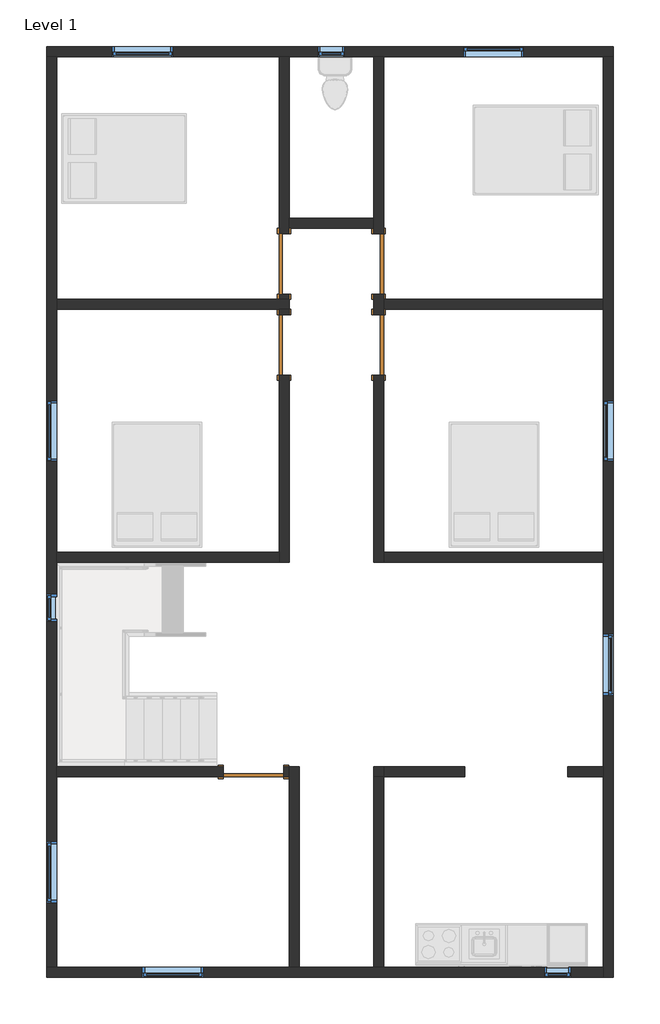
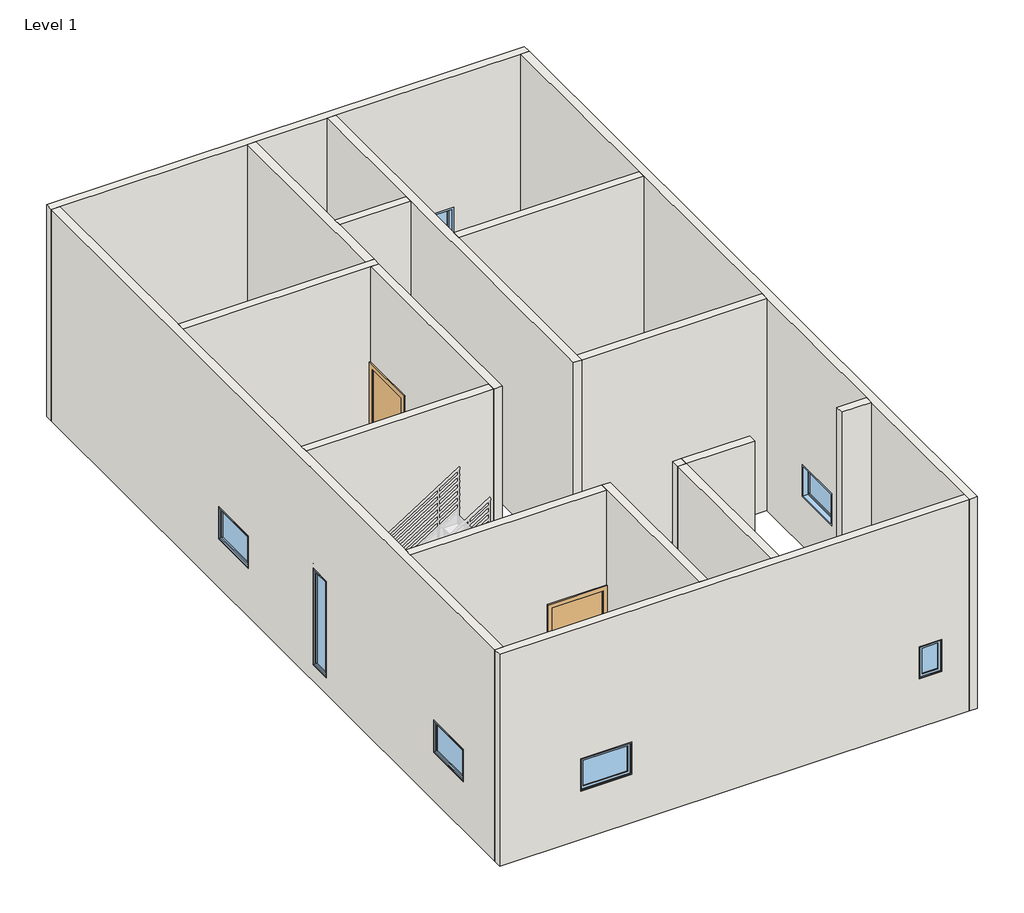
# One storey, part 1 of 4: 18 walls, 10 windows, 5 doors.
"""IFC4 building model written with IfcOpenShell, lengths in millimetres."""

from ifc_helpers import new_model, si_unit, frame, origin, origin_with_axes, place, context, project, spatial, polyline, outline, extrude, faceted_brep, transform, mapped, element, save
from components import m_single_flush_0915_x_2134mm_f3d7f739, m_single_flush_0915_x_2134mm_138fd904, m_fixed_0406_x_0610mm_893b2dd9, m_fixed_0406_x_1830mm_a81fa326, m_fixed_0915_x_0610mm_ad787ded

model = new_model("IFC4")

# Units and contexts
model_context = context("Model", 3, world=origin())
ifc_project = project(units=[si_unit("LENGTHUNIT", "METRE", prefix="MILLI")], contexts=[model_context])

# Site, building, storey
site = spatial("IfcSite", under=ifc_project)
building = spatial("IfcBuilding", under=site)
storey = spatial("IfcBuildingStorey", under=building, Name="Level 1", Elevation=0.0)

# Doors
placement = place(None, origin())
m_single_flush_0915_x_2134mm_shape = m_single_flush_0915_x_2134mm_f3d7f739(model_context)
element("IfcDoor", 1, ObjectType="M_Single-Flush : 0915 x 2134mm", at=placement, inside=storey, context=model_context, shape_type="MappedRepresentation", body=[
    mapped(m_single_flush_0915_x_2134mm_shape, transform((-9575.5381184, 8355.0527383, 0.0), x_axis=(0.0, -1.0, 0.0), y_axis=(1.0, 0.0, 0.0), z_axis=(0.0, 0.0, 1.0))),
])
element("IfcDoor", 2, ObjectType="M_Single-Flush : 0915 x 2134mm", at=placement, inside=storey, context=model_context, shape_type="MappedRepresentation", body=[
    mapped(m_single_flush_0915_x_2134mm_shape, transform((-8151.9381184, 7135.5527383, 0.0), x_axis=(0.0, 1.0, 0.0), y_axis=(-1.0, 0.0, 0.0), z_axis=(0.0, 0.0, 1.0))),
])
element("IfcDoor", 3, ObjectType="M_Single-Flush : 0915 x 2134mm", at=placement, inside=storey, context=model_context, shape_type="MappedRepresentation", body=[
    mapped(m_single_flush_0915_x_2134mm_shape, transform((-10035.1381184, 703.3527383, 0.0), x_axis=(1.0, 0.0, 0.0), y_axis=(0.0, 1.0, 0.0), z_axis=(0.0, 0.0, 1.0))),
])
m_single_flush_0915_x_2134mm_2_shape = m_single_flush_0915_x_2134mm_138fd904(model_context)
element("IfcDoor", 4, ObjectType="M_Single-Flush : 0915 x 2134mm", at=placement, inside=storey, context=model_context, shape_type="MappedRepresentation", body=[
    mapped(m_single_flush_0915_x_2134mm_2_shape, transform((-8151.9381184, 8355.0527383, 0.0), x_axis=(0.0, -1.0, 0.0), y_axis=(1.0, 0.0, 0.0), z_axis=(0.0, 0.0, 1.0))),
])
element("IfcDoor", 5, ObjectType="M_Single-Flush : 0915 x 2134mm", at=placement, inside=storey, context=model_context, shape_type="MappedRepresentation", body=[
    mapped(m_single_flush_0915_x_2134mm_2_shape, transform((-9575.5381184, 7135.5527383, 0.0), x_axis=(0.0, 1.0, 0.0), y_axis=(-1.0, 0.0, 0.0), z_axis=(0.0, 0.0, 1.0))),
])

# Walls
element("IfcWall", 6, ObjectType="Generic - 150mm", at=placement, inside=storey, context=model_context, shape_type="Brep", body=[
    faceted_brep([(-13153.3381184, 11478.9527383, 0.0), (-13003.3381184, 11478.9527383, 0.0), (-9650.5381184, 11478.9527383, 0.0), (-9500.5381184, 11478.9527383, 0.0), (-8226.9381184, 11478.9527383, 0.0), (-8076.9381184, 11478.9527383, 0.0), (-4768.9381184, 11478.9527383, 0.0), (-4618.9381184, 11478.9527383, 0.0), (-4618.9381184, 11478.9527383, 4000.0), (-4768.9381184, 11478.9527383, 4000.0), (-8076.9381184, 11478.9527383, 4000.0), (-8226.9381184, 11478.9527383, 4000.0), (-9500.5381184, 11478.9527383, 4000.0), (-9650.5381184, 11478.9527383, 4000.0), (-13003.3381184, 11478.9527383, 4000.0), (-13153.3381184, 11478.9527383, 4000.0), (-8660.7381184, 11478.9527383, 915.0), (-9066.7381184, 11478.9527383, 915.0), (-9066.7381184, 11478.9527383, 1525.0), (-8660.7381184, 11478.9527383, 1525.0), (-6880.4381184, 11478.9527383, 915.0), (-6880.4381184, 11478.9527383, 1525.0), (-5965.4381184, 11478.9527383, 1525.0), (-5965.4381184, 11478.9527383, 915.0), (-11249.2381184, 11478.9527383, 915.0), (-12164.2381184, 11478.9527383, 915.0), (-12164.2381184, 11478.9527383, 1525.0), (-11249.2381184, 11478.9527383, 1525.0), (-13153.3381184, 11628.9527383, 0.0), (-13153.3381184, 11628.9527383, 4000.0), (-4618.9381184, 11628.9527383, 4000.0), (-4618.9381184, 11628.9527383, 0.0), (-8660.7381184, 11628.9527383, 915.0), (-8660.7381184, 11628.9527383, 1525.0), (-9066.7381184, 11628.9527383, 1525.0), (-9066.7381184, 11628.9527383, 915.0), (-6880.4381184, 11628.9527383, 915.0), (-5965.4381184, 11628.9527383, 915.0), (-5965.4381184, 11628.9527383, 1525.0), (-6880.4381184, 11628.9527383, 1525.0), (-11249.2381184, 11628.9527383, 915.0), (-11249.2381184, 11628.9527383, 1525.0), (-12164.2381184, 11628.9527383, 1525.0), (-12164.2381184, 11628.9527383, 915.0)], [[[0, 1, 2, 3, 4, 5, 6, 7, 8, 9, 10, 11, 12, 13, 14, 15], [16, 17, 18, 19], [20, 21, 22, 23], [24, 25, 26, 27]], [[28, 29, 30, 31], [32, 33, 34, 35], [36, 37, 38, 39], [40, 41, 42, 43]], [[7, 6, 5, 4, 3, 2, 1, 0, 28, 31]], [[15, 14, 13, 12, 11, 10, 9, 8, 30, 29]], [[8, 7, 31, 30]], [[0, 15, 29, 28]], [[33, 32, 16, 19]], [[34, 33, 19, 18]], [[35, 34, 18, 17]], [[32, 35, 17, 16]], [[21, 20, 36, 39]], [[22, 21, 39, 38]], [[23, 22, 38, 37]], [[20, 23, 37, 36]], [[41, 40, 24, 27]], [[42, 41, 27, 26]], [[43, 42, 26, 25]], [[40, 43, 25, 24]]]),
])
element("IfcWall", 7, ObjectType="Generic - 150mm", at=placement, inside=storey, context=model_context, shape_type="Brep", body=[
    faceted_brep([(-4768.9381184, 11478.9527383, 0.0), (-4768.9381184, 7820.1527383, 0.0), (-4768.9381184, 7670.1527383, 0.0), (-4768.9381184, 4010.1527383, 0.0), (-4768.9381184, 3860.1527383, 0.0), (-4768.9381184, 778.3527383, 0.0), (-4768.9381184, 628.3527383, 0.0), (-4768.9381184, -2241.8472617, 0.0), (-4768.9381184, -2391.8472617, 0.0), (-4768.9381184, -2391.8472617, 4000.0), (-4768.9381184, -2241.8472617, 4000.0), (-4768.9381184, 628.3527383, 4000.0), (-4768.9381184, 778.3527383, 4000.0), (-4768.9381184, 3860.1527383, 4000.0), (-4768.9381184, 4010.1527383, 4000.0), (-4768.9381184, 7670.1527383, 4000.0), (-4768.9381184, 7820.1527383, 4000.0), (-4768.9381184, 11478.9527383, 4000.0), (-4768.9381184, 2776.7527383, 915.0), (-4768.9381184, 2776.7527383, 1525.0), (-4768.9381184, 1861.7527383, 1525.0), (-4768.9381184, 1861.7527383, 915.0), (-4768.9381184, 5382.6527383, 915.0), (-4768.9381184, 6297.6527383, 915.0), (-4768.9381184, 6297.6527383, 1525.0), (-4768.9381184, 5382.6527383, 1525.0), (-4618.9381184, 11478.9527383, 0.0), (-4618.9381184, 11478.9527383, 4000.0), (-4618.9381184, -2391.8472617, 4000.0), (-4618.9381184, -2391.8472617, 0.0), (-4618.9381184, 2776.7527383, 915.0), (-4618.9381184, 1861.7527383, 915.0), (-4618.9381184, 1861.7527383, 1525.0), (-4618.9381184, 2776.7527383, 1525.0), (-4618.9381184, 5382.6527383, 915.0), (-4618.9381184, 5382.6527383, 1525.0), (-4618.9381184, 6297.6527383, 1525.0), (-4618.9381184, 6297.6527383, 915.0)], [[[0, 1, 2, 3, 4, 5, 6, 7, 8, 9, 10, 11, 12, 13, 14, 15, 16, 17], [18, 19, 20, 21], [22, 23, 24, 25]], [[26, 27, 28, 29], [30, 31, 32, 33], [34, 35, 36, 37]], [[8, 7, 6, 5, 4, 3, 2, 1, 0, 26, 29]], [[17, 16, 15, 14, 13, 12, 11, 10, 9, 28, 27]], [[0, 17, 27, 26]], [[9, 8, 29, 28]], [[19, 18, 30, 33]], [[20, 19, 33, 32]], [[21, 20, 32, 31]], [[18, 21, 31, 30]], [[35, 34, 22, 25]], [[36, 35, 25, 24]], [[37, 36, 24, 23]], [[34, 37, 23, 22]]]),
])
element("IfcWall", 8, ObjectType="Generic - 150mm", at=placement, inside=storey, context=model_context, shape_type="Brep", body=[
    faceted_brep([(-4768.9381184, -2241.8472617, 0.0), (-8076.9381184, -2241.8472617, 0.0), (-8226.9381184, -2241.8472617, 0.0), (-9350.5381184, -2241.8472617, 0.0), (-9500.5381184, -2241.8472617, 0.0), (-13003.3381184, -2241.8472617, 0.0), (-13153.3381184, -2241.8472617, 0.0), (-13153.3381184, -2241.8472617, 4000.0), (-13003.3381184, -2241.8472617, 4000.0), (-9500.5381184, -2241.8472617, 4000.0), (-9350.5381184, -2241.8472617, 4000.0), (-8226.9381184, -2241.8472617, 4000.0), (-8076.9381184, -2241.8472617, 4000.0), (-4768.9381184, -2241.8472617, 4000.0), (-5252.9381184, -2241.8472617, 915.0), (-5252.9381184, -2241.8472617, 1525.0), (-5658.9381184, -2241.8472617, 1525.0), (-5658.9381184, -2241.8472617, 915.0), (-10794.4381184, -2241.8472617, 915.0), (-10794.4381184, -2241.8472617, 1525.0), (-11709.4381184, -2241.8472617, 1525.0), (-11709.4381184, -2241.8472617, 915.0), (-4768.9381184, -2391.8472617, 0.0), (-4768.9381184, -2391.8472617, 4000.0), (-13153.3381184, -2391.8472617, 4000.0), (-13153.3381184, -2391.8472617, 0.0), (-5252.9381184, -2391.8472617, 915.0), (-5658.9381184, -2391.8472617, 915.0), (-5658.9381184, -2391.8472617, 1525.0), (-5252.9381184, -2391.8472617, 1525.0), (-10794.4381184, -2391.8472617, 915.0), (-11709.4381184, -2391.8472617, 915.0), (-11709.4381184, -2391.8472617, 1525.0), (-10794.4381184, -2391.8472617, 1525.0)], [[[0, 1, 2, 3, 4, 5, 6, 7, 8, 9, 10, 11, 12, 13], [14, 15, 16, 17], [18, 19, 20, 21]], [[22, 23, 24, 25], [26, 27, 28, 29], [30, 31, 32, 33]], [[6, 5, 4, 3, 2, 1, 0, 22, 25]], [[13, 12, 11, 10, 9, 8, 7, 24, 23]], [[0, 13, 23, 22]], [[7, 6, 25, 24]], [[15, 14, 26, 29]], [[16, 15, 29, 28]], [[17, 16, 28, 27]], [[14, 17, 27, 26]], [[19, 18, 30, 33]], [[20, 19, 33, 32]], [[21, 20, 32, 31]], [[18, 21, 31, 30]]]),
])
element("IfcWall", 9, ObjectType="Generic - 150mm", at=placement, inside=storey, context=model_context, shape_type="Brep", body=[
    faceted_brep([(-13003.3381184, -2241.8472617, 0.0), (-13003.3381184, 628.3527383, 0.0), (-13003.3381184, 778.3527383, 0.0), (-13003.3381184, 3860.1527383, 0.0), (-13003.3381184, 4010.1527383, 0.0), (-13003.3381184, 7670.1527383, 0.0), (-13003.3381184, 7820.1527383, 0.0), (-13003.3381184, 11478.9527383, 0.0), (-13003.3381184, 11478.9527383, 4000.0), (-13003.3381184, 7820.1527383, 4000.0), (-13003.3381184, 7670.1527383, 4000.0), (-13003.3381184, 4010.1527383, 4000.0), (-13003.3381184, 3860.1527383, 4000.0), (-13003.3381184, 778.3527383, 4000.0), (-13003.3381184, 628.3527383, 4000.0), (-13003.3381184, -2241.8472617, 4000.0), (-13003.3381184, -1264.2472617, 915.0), (-13003.3381184, -1264.2472617, 1525.0), (-13003.3381184, -349.2472617, 1525.0), (-13003.3381184, -349.2472617, 915.0), (-13003.3381184, 5382.6527383, 915.0), (-13003.3381184, 5382.6527383, 1525.0), (-13003.3381184, 6297.6527383, 1525.0), (-13003.3381184, 6297.6527383, 915.0), (-13003.3381184, 2970.1527383, 305.0), (-13003.3381184, 2970.1527383, 2135.0), (-13003.3381184, 3376.1527383, 2135.0), (-13003.3381184, 3376.1527383, 305.0), (-13153.3381184, -2241.8472617, 0.0), (-13153.3381184, -2241.8472617, 4000.0), (-13153.3381184, 11478.9527383, 4000.0), (-13153.3381184, 11478.9527383, 0.0), (-13153.3381184, -1264.2472617, 915.0), (-13153.3381184, -349.2472617, 915.0), (-13153.3381184, -349.2472617, 1525.0), (-13153.3381184, -1264.2472617, 1525.0), (-13153.3381184, 5382.6527383, 915.0), (-13153.3381184, 6297.6527383, 915.0), (-13153.3381184, 6297.6527383, 1525.0), (-13153.3381184, 5382.6527383, 1525.0), (-13153.3381184, 2970.1527383, 305.0), (-13153.3381184, 3376.1527383, 305.0), (-13153.3381184, 3376.1527383, 2135.0), (-13153.3381184, 2970.1527383, 2135.0)], [[[0, 1, 2, 3, 4, 5, 6, 7, 8, 9, 10, 11, 12, 13, 14, 15], [16, 17, 18, 19], [20, 21, 22, 23], [24, 25, 26, 27]], [[28, 29, 30, 31], [32, 33, 34, 35], [36, 37, 38, 39], [40, 41, 42, 43]], [[7, 6, 5, 4, 3, 2, 1, 0, 28, 31]], [[15, 14, 13, 12, 11, 10, 9, 8, 30, 29]], [[0, 15, 29, 28]], [[8, 7, 31, 30]], [[17, 16, 32, 35]], [[18, 17, 35, 34]], [[19, 18, 34, 33]], [[16, 19, 33, 32]], [[21, 20, 36, 39]], [[22, 21, 39, 38]], [[23, 22, 38, 37]], [[20, 23, 37, 36]], [[25, 24, 40, 43]], [[26, 25, 43, 42]], [[27, 26, 42, 41]], [[24, 27, 41, 40]]]),
])
element("IfcWall", 10, ObjectType="Generic - 150mm", at=placement, inside=storey, context=model_context, shape_type="Brep", body=[
    faceted_brep([(-13003.3381184, 7670.1527383, 0.0), (-9650.5381184, 7670.1527383, 0.0), (-9500.5381184, 7670.1527383, 0.0), (-9500.5381184, 7670.1527383, 4000.0), (-9650.5381184, 7670.1527383, 4000.0), (-13003.3381184, 7670.1527383, 4000.0), (-13003.3381184, 7820.1527383, 0.0), (-13003.3381184, 7820.1527383, 4000.0), (-9650.5381184, 7820.1527383, 4000.0), (-9500.5381184, 7820.1527383, 4000.0), (-9500.5381184, 7820.1527383, 0.0), (-9650.5381184, 7820.1527383, 0.0)], [[[0, 1, 2, 3, 4, 5]], [[6, 7, 8, 9, 10, 11]], [[2, 1, 0, 6, 11, 10]], [[5, 4, 3, 9, 8, 7]], [[0, 5, 7, 6]], [[3, 2, 10, 9]]]),
])
element("IfcWall", 11, ObjectType="Generic - 150mm", at=placement, inside=storey, context=model_context, shape_type="Brep", body=[
    faceted_brep([(-9500.5381184, 7820.1527383, 0.0), (-9500.5381184, 7897.5527383, 0.0), (-9500.5381184, 7897.5527383, 2134.0), (-9500.5381184, 8812.5527383, 2134.0), (-9500.5381184, 8812.5527383, 0.0), (-9500.5381184, 8889.9527383, 0.0), (-9500.5381184, 9039.9527383, 0.0), (-9500.5381184, 11478.9527383, 0.0), (-9500.5381184, 11478.9527383, 4000.0), (-9500.5381184, 9039.9527383, 4000.0), (-9500.5381184, 8889.9527383, 4000.0), (-9500.5381184, 7820.1527383, 4000.0), (-9650.5381184, 7897.5527383, 2134.0), (-9650.5381184, 7897.5527383, 0.0), (-9650.5381184, 7820.1527383, 0.0), (-9650.5381184, 7820.1527383, 4000.0), (-9650.5381184, 11478.9527383, 4000.0), (-9650.5381184, 11478.9527383, 0.0), (-9650.5381184, 8812.5527383, 0.0), (-9650.5381184, 8812.5527383, 2134.0)], [[[0, 1, 2, 3, 4, 5, 6, 7, 8, 9, 10, 11]], [[12, 13, 14, 15, 16, 17, 18, 19]], [[18, 17, 7, 6, 5, 4]], [[14, 13, 1, 0]], [[11, 10, 9, 8, 16, 15]], [[0, 11, 15, 14]], [[8, 7, 17, 16]], [[2, 1, 13, 12]], [[3, 2, 12, 19]], [[4, 3, 19, 18]]]),
])
element("IfcWall", 12, ObjectType="Generic - 150mm", at=placement, inside=storey, context=model_context, shape_type="Brep", body=[
    faceted_brep([(-8226.9381184, 7897.5527383, 0.0), (-8226.9381184, 7593.0527383, 0.0), (-8226.9381184, 7593.0527383, 2134.0), (-8226.9381184, 6678.0527383, 2134.0), (-8226.9381184, 6678.0527383, 0.0), (-8226.9381184, 3860.1527383, 0.0), (-8226.9381184, 3860.1527383, 4000.0), (-8226.9381184, 8889.9527383, 4000.0), (-8226.9381184, 9039.9527383, 4000.0), (-8226.9381184, 11478.9527383, 4000.0), (-8226.9381184, 11478.9527383, 0.0), (-8226.9381184, 9039.9527383, 0.0), (-8226.9381184, 8889.9527383, 0.0), (-8226.9381184, 8812.5527383, 0.0), (-8226.9381184, 8812.5527383, 2134.0), (-8226.9381184, 7897.5527383, 2134.0), (-8076.9381184, 7593.0527383, 2134.0), (-8076.9381184, 7593.0527383, 0.0), (-8076.9381184, 7670.1527383, 0.0), (-8076.9381184, 7820.1527383, 0.0), (-8076.9381184, 7897.5527383, 0.0), (-8076.9381184, 7897.5527383, 2134.0), (-8076.9381184, 8812.5527383, 2134.0), (-8076.9381184, 8812.5527383, 0.0), (-8076.9381184, 11478.9527383, 0.0), (-8076.9381184, 11478.9527383, 4000.0), (-8076.9381184, 7820.1527383, 4000.0), (-8076.9381184, 7670.1527383, 4000.0), (-8076.9381184, 4010.1527383, 4000.0), (-8076.9381184, 3860.1527383, 4000.0), (-8076.9381184, 3860.1527383, 0.0), (-8076.9381184, 4010.1527383, 0.0), (-8076.9381184, 6678.0527383, 0.0), (-8076.9381184, 6678.0527383, 2134.0)], [[[0, 1, 2, 3, 4, 5, 6, 7, 8, 9, 10, 11, 12, 13, 14, 15]], [[16, 17, 18, 19, 20, 21, 22, 23, 24, 25, 26, 27, 28, 29, 30, 31, 32, 33]], [[13, 12, 11, 10, 24, 23]], [[32, 31, 30, 5, 4]], [[20, 19, 18, 17, 1, 0]], [[9, 8, 7, 6, 29, 28, 27, 26, 25]], [[10, 9, 25, 24]], [[21, 20, 0, 15]], [[22, 21, 15, 14]], [[23, 22, 14, 13]], [[6, 5, 30, 29]], [[2, 1, 17, 16]], [[3, 2, 16, 33]], [[4, 3, 33, 32]]]),
])
element("IfcWall", 13, ObjectType="Generic - 150mm", at=placement, inside=storey, context=model_context, shape_type="SweptSolid", body=[
    extrude(outline(polyline([(-4768.9381184, 7670.1527383), (-8076.9381184, 7670.1527383), (-8076.9381184, 7820.1527383), (-4768.9381184, 7820.1527383), (-4768.9381184, 7670.1527383)])), origin_with_axes(), (0.0, 0.0, 1.0), 4000.0),
])
element("IfcWall", 14, ObjectType="Generic - 150mm", at=placement, inside=storey, context=model_context, shape_type="SweptSolid", body=[
    extrude(outline(polyline([(-8226.9381184, 8889.9527383), (-9500.5381184, 8889.9527383), (-9500.5381184, 9039.9527383), (-8226.9381184, 9039.9527383), (-8226.9381184, 8889.9527383)])), origin_with_axes(), (0.0, 0.0, 1.0), 4000.0),
])
element("IfcWall", 15, ObjectType="Generic - 150mm", at=placement, inside=storey, context=model_context, shape_type="Brep", body=[
    faceted_brep([(-9650.5381184, 7670.1527383, 0.0), (-9650.5381184, 7593.0527383, 0.0), (-9650.5381184, 7593.0527383, 2134.0), (-9650.5381184, 6678.0527383, 2134.0), (-9650.5381184, 6678.0527383, 0.0), (-9650.5381184, 4010.1527383, 0.0), (-9650.5381184, 3860.1527383, 0.0), (-9650.5381184, 3860.1527383, 4000.0), (-9650.5381184, 4010.1527383, 4000.0), (-9650.5381184, 7670.1527383, 4000.0), (-9500.5381184, 7593.0527383, 2134.0), (-9500.5381184, 7593.0527383, 0.0), (-9500.5381184, 7670.1527383, 0.0), (-9500.5381184, 7670.1527383, 4000.0), (-9500.5381184, 3860.1527383, 4000.0), (-9500.5381184, 3860.1527383, 0.0), (-9500.5381184, 6678.0527383, 0.0), (-9500.5381184, 6678.0527383, 2134.0)], [[[0, 1, 2, 3, 4, 5, 6, 7, 8, 9]], [[10, 11, 12, 13, 14, 15, 16, 17]], [[16, 15, 6, 5, 4]], [[12, 11, 1, 0]], [[9, 8, 7, 14, 13]], [[0, 9, 13, 12]], [[7, 6, 15, 14]], [[2, 1, 11, 10]], [[3, 2, 10, 17]], [[4, 3, 17, 16]]]),
])
element("IfcWall", 16, ObjectType="Generic - 150mm", at=placement, inside=storey, context=model_context, shape_type="SweptSolid", body=[
    extrude(outline(polyline([(-13003.3381184, 4010.1527383), (-9650.5381184, 4010.1527383), (-9650.5381184, 3860.1527383), (-13003.3381184, 3860.1527383), (-13003.3381184, 4010.1527383)])), origin_with_axes(), (0.0, 0.0, 1.0), 4000.0),
])
element("IfcWall", 17, ObjectType="Generic - 150mm", at=placement, inside=storey, context=model_context, shape_type="SweptSolid", body=[
    extrude(outline(polyline([(-4768.9381184, 3860.1527383), (-8076.9381184, 3860.1527383), (-8076.9381184, 4010.1527383), (-4768.9381184, 4010.1527383), (-4768.9381184, 3860.1527383)])), origin_with_axes(), (0.0, 0.0, 1.0), 4000.0),
])
element("IfcWall", 18, ObjectType="Generic - 150mm", at=placement, inside=storey, context=model_context, shape_type="Brep", body=[
    faceted_brep([(-9350.5381184, -2241.8472617, 0.0), (-9350.5381184, 778.3527383, 0.0), (-9350.5381184, 778.3527383, 4000.0), (-9350.5381184, -2241.8472617, 4000.0), (-9500.5381184, -2241.8472617, 0.0), (-9500.5381184, -2241.8472617, 4000.0), (-9500.5381184, 628.3527383, 4000.0), (-9500.5381184, 778.3527383, 4000.0), (-9500.5381184, 778.3527383, 0.0), (-9500.5381184, 628.3527383, 0.0)], [[[0, 1, 2, 3]], [[4, 5, 6, 7, 8, 9]], [[1, 0, 4, 9, 8]], [[3, 2, 7, 6, 5]], [[0, 3, 5, 4]], [[2, 1, 8, 7]]]),
])
element("IfcWall", 19, ObjectType="Generic - 150mm", at=placement, inside=storey, context=model_context, shape_type="SweptSolid", body=[
    extrude(outline(polyline([(2134.0, -9577.6381184), (0.0, -9577.6381184), (0.0, -9500.5381184), (4000.0, -9500.5381184), (4000.0, -13003.3381184), (0.0, -13003.3381184), (0.0, -10492.6381184), (2134.0, -10492.6381184), (2134.0, -9577.6381184)])), frame((0.0, 628.3527383, 0.0), z_axis=(0.0, 1.0, 0.0), x_axis=(0.0, 0.0, 1.0)), (0.0, 0.0, 1.0), 150.0),
])
element("IfcWall", 20, ObjectType="Generic - 150mm", at=placement, inside=storey, context=model_context, shape_type="SweptSolid", body=[
    extrude(outline(polyline([(-8226.9381184, -2241.8472617), (-8226.9381184, 628.3527383), (-8076.9381184, 628.3527383), (-8076.9381184, -2241.8472617), (-8226.9381184, -2241.8472617)])), origin_with_axes(), (0.0, 0.0, 1.0), 4000.0),
])
element("IfcWall", 21, ObjectType="Generic - 150mm", at=placement, inside=storey, context=model_context, shape_type="Brep", body=[
    faceted_brep([(-8076.9381184, 628.3527383, 0.0), (-8076.9381184, 630.7527383, 0.0), (-8076.9381184, 780.7527383, 0.0), (-8076.9381184, 780.7527383, 4000.0), (-8076.9381184, 630.7527383, 4000.0), (-8076.9381184, 628.3527383, 4000.0), (-8226.9381184, 628.3527383, 0.0), (-8226.9381184, 628.3527383, 4000.0), (-8226.9381184, 780.7527383, 4000.0), (-8226.9381184, 780.7527383, 0.0)], [[[0, 1, 2, 3, 4, 5]], [[6, 7, 8, 9]], [[2, 1, 0, 6, 9]], [[5, 4, 3, 8, 7]], [[0, 5, 7, 6]], [[3, 2, 9, 8]]]),
])
element("IfcWall", 22, ObjectType="Generic - 150mm", at=placement, inside=storey, context=model_context, shape_type="SweptSolid", body=[
    extrude(outline(polyline([(-6855.3381184, 630.7527383), (-8076.9381184, 630.7527383), (-8076.9381184, 780.7527383), (-6855.3381184, 780.7527383), (-6855.3381184, 630.7527383)])), origin_with_axes(), (0.0, 0.0, 1.0), 4000.0),
])
element("IfcWall", 23, ObjectType="Generic - 150mm", at=placement, inside=storey, context=model_context, shape_type="SweptSolid", body=[
    extrude(outline(polyline([(-5303.5381184, 778.3527383), (-4768.9381184, 778.3527383), (-4768.9381184, 628.3527383), (-5303.5381184, 628.3527383), (-5303.5381184, 778.3527383)])), origin_with_axes(), (0.0, 0.0, 1.0), 4000.0),
])

# Windows
m_fixed_0406_x_0610mm_shape = m_fixed_0406_x_0610mm_893b2dd9(model_context)
element("IfcWindow", 24, ObjectType="M_Fixed : 0406 x 0610mm", at=placement, inside=storey, context=model_context, shape_type="MappedRepresentation", body=[
    mapped(m_fixed_0406_x_0610mm_shape, transform((-8863.7381184, 11566.9527383, 0.0), x_axis=(-1.0, 0.0, 0.0), y_axis=(0.0, -1.0, 0.0), z_axis=(0.0, 0.0, 1.0))),
])
element("IfcWindow", 25, ObjectType="M_Fixed : 0406 x 0610mm", at=placement, inside=storey, context=model_context, shape_type="MappedRepresentation", body=[
    mapped(m_fixed_0406_x_0610mm_shape, transform((-5455.9381184, -2303.8472617, 0.0), x_axis=(-1.0, 0.0, 0.0), y_axis=(0.0, -1.0, 0.0), z_axis=(0.0, 0.0, 1.0))),
])
m_fixed_0406_x_1830mm_shape = m_fixed_0406_x_1830mm_a81fa326(model_context)
element("IfcWindow", 26, ObjectType="M_Fixed : 0406 x 1830mm", at=placement, inside=storey, context=model_context, shape_type="MappedRepresentation", body=[
    mapped(m_fixed_0406_x_1830mm_shape, transform((-13065.3381184, 3173.1527383, 0.0), x_axis=(0.0, 1.0, 0.0), y_axis=(-1.0, 0.0, 0.0), z_axis=(0.0, 0.0, 1.0))),
])
m_fixed_0915_x_0610mm_shape = m_fixed_0915_x_0610mm_ad787ded(model_context)
element("IfcWindow", 27, ObjectType="M_Fixed : 0915 x 0610mm", at=placement, inside=storey, context=model_context, shape_type="MappedRepresentation", body=[
    mapped(m_fixed_0915_x_0610mm_shape, transform((-11251.9381184, -2303.8472617, 0.0), x_axis=(-1.0, 0.0, 0.0), y_axis=(0.0, -1.0, 0.0), z_axis=(0.0, 0.0, 1.0))),
])
element("IfcWindow", 28, ObjectType="M_Fixed : 0915 x 0610mm", at=placement, inside=storey, context=model_context, shape_type="MappedRepresentation", body=[
    mapped(m_fixed_0915_x_0610mm_shape, transform((-13065.3381184, -806.7472617, 0.0), x_axis=(0.0, 1.0, 0.0), y_axis=(-1.0, 0.0, 0.0), z_axis=(0.0, 0.0, 1.0))),
])
element("IfcWindow", 29, ObjectType="M_Fixed : 0915 x 0610mm", at=placement, inside=storey, context=model_context, shape_type="MappedRepresentation", body=[
    mapped(m_fixed_0915_x_0610mm_shape, transform((-4706.9381184, 2319.2527383, 0.0), x_axis=(0.0, -1.0, 0.0), y_axis=(1.0, 0.0, 0.0), z_axis=(0.0, 0.0, 1.0))),
])
element("IfcWindow", 30, ObjectType="M_Fixed : 0915 x 0610mm", at=placement, inside=storey, context=model_context, shape_type="MappedRepresentation", body=[
    mapped(m_fixed_0915_x_0610mm_shape, transform((-13065.3381184, 5840.1527383, 0.0), x_axis=(0.0, 1.0, 0.0), y_axis=(-1.0, 0.0, 0.0), z_axis=(0.0, 0.0, 1.0))),
])
element("IfcWindow", 31, ObjectType="M_Fixed : 0915 x 0610mm", at=placement, inside=storey, context=model_context, shape_type="MappedRepresentation", body=[
    mapped(m_fixed_0915_x_0610mm_shape, transform((-4680.9381184, 5840.1527383, 0.0), x_axis=(0.0, 1.0, 0.0), y_axis=(-1.0, 0.0, 0.0), z_axis=(0.0, 0.0, 1.0))),
])
element("IfcWindow", 32, ObjectType="M_Fixed : 0915 x 0610mm", at=placement, inside=storey, context=model_context, shape_type="MappedRepresentation", body=[
    mapped(m_fixed_0915_x_0610mm_shape, transform((-6422.9381184, 11540.9527383, 0.0), x_axis=(1.0, 0.0, 0.0), y_axis=(0.0, 1.0, 0.0), z_axis=(0.0, 0.0, 1.0))),
])
element("IfcWindow", 33, ObjectType="M_Fixed : 0915 x 0610mm", at=placement, inside=storey, context=model_context, shape_type="MappedRepresentation", body=[
    mapped(m_fixed_0915_x_0610mm_shape, transform((-11706.7381184, 11566.9527383, 0.0), x_axis=(-1.0, 0.0, 0.0), y_axis=(0.0, -1.0, 0.0), z_axis=(0.0, 0.0, 1.0))),
])

save(model, "model.ifc")

# Revit data of these elements
# Type "M_Single-Flush : 0915 x 2134mm"
#   Type Mark = "15"
#   Thickness = 51 mm
#   Height = 2134 mm
#   Trim Projection Ext = 25 mm
#   Trim Projection Int = 25 mm
#   Trim Width = 76 mm
#   Width = 915 mm
#   Door Material = Door - Panel
#   Frame Material = Door - Frame
#   Function = (empty or 0)
#   Wall Closure = (empty or 0)
# Type "Generic - 150mm"
#   Layers, outside or top first: 150 mm no material (function 1)
# Type "M_Fixed : 0406 x 0610mm"
#   Type Mark = "10"
#   Height = 610 mm
#   Default Sill Height = 915 mm
#   Width = 406 mm
#   Window Inset = 19 mm
#   Frame Exterior Material = Sash
#   Frame Interior Material = Sash
#   Glass Pane Material = Glass
#   Sash = Sash
#   Wall Closure = (empty or 0)
# Type "M_Fixed : 0406 x 1830mm"
#   Type Mark = "16"
#   Height = 1830 mm
#   Default Sill Height = 305 mm
#   Width = 406 mm
#   Window Inset = 19 mm
#   Frame Exterior Material = Sash
#   Frame Interior Material = Sash
#   Glass Pane Material = Glass
#   Sash = Sash
#   Wall Closure = (empty or 0)
# Type "M_Fixed : 0915 x 0610mm"
#   Type Mark = "14"
#   Height = 610 mm
#   Default Sill Height = 915 mm
#   Width = 915 mm
#   Window Inset = 19 mm
#   Frame Exterior Material = Sash
#   Frame Interior Material = Sash
#   Glass Pane Material = Glass
#   Sash = Sash
#   Wall Closure = (empty or 0)
# Elements 1, 2, 3, 4, 5 (IfcDoor, "M_Single-Flush : 0915 x 2134mm")
#   Phase Created = New Construction
#   Materials on its faces: "Door - Frame", "Door - Panel"
# Elements 6, 7, 8, 9, 10, 11, 12, 13, 14, 15, 16, 17, 18, 19, 20, 21, 22, 23 (IfcWall, "Generic - 150mm")
#   Top Offset = 0 mm
#   Base Offset = 0 mm
#   wall height = 4000 mm
#   Phase Created = New Construction
#   Base Constraint = Level 1
#   Top Constraint = Level 2
#   Materials on its faces: "Default Wall"
# Element 24 (IfcWindow, "M_Fixed : 0406 x 0610mm")
#   Mark = "6"
#   Phase Created = New Construction
#   Materials on its faces: "Sash", "Glass"
# Element 25 (IfcWindow, "M_Fixed : 0406 x 0610mm")
#   Mark = "7"
#   Phase Created = New Construction
#   Materials on its faces: "Sash", "Glass"
# Element 26 (IfcWindow, "M_Fixed : 0406 x 1830mm")
#   Mark = "15"
#   Phase Created = New Construction
#   Materials on its faces: "Sash", "Glass"
# Element 27 (IfcWindow, "M_Fixed : 0915 x 0610mm")
#   Mark = "8"
#   Phase Created = New Construction
#   Materials on its faces: "Sash", "Glass"
# Element 28 (IfcWindow, "M_Fixed : 0915 x 0610mm")
#   Mark = "9"
#   Phase Created = New Construction
#   Materials on its faces: "Sash", "Glass"
# Element 29 (IfcWindow, "M_Fixed : 0915 x 0610mm")
#   Mark = "10"
#   Phase Created = New Construction
#   Materials on its faces: "Sash", "Glass"
# Element 30 (IfcWindow, "M_Fixed : 0915 x 0610mm")
#   Mark = "11"
#   Phase Created = New Construction
#   Materials on its faces: "Sash", "Glass"
# Element 31 (IfcWindow, "M_Fixed : 0915 x 0610mm")
#   Mark = "12"
#   Phase Created = New Construction
#   Materials on its faces: "Sash", "Glass"
# Element 32 (IfcWindow, "M_Fixed : 0915 x 0610mm")
#   Mark = "13"
#   Phase Created = New Construction
#   Materials on its faces: "Sash", "Glass"
# Element 33 (IfcWindow, "M_Fixed : 0915 x 0610mm")
#   Mark = "14"
#   Phase Created = New Construction
#   Materials on its faces: "Sash", "Glass"
# Materials
#   "Door - Panel": class "Wood", colour RGB 114 82 51, transparency 0
#   "Door - Frame": colour RGB 153 76 43, transparency 0
#   "Sash": class "Wood", colour RGB 136 99 55, transparency 0
#   "Glass": class "Glass", colour RGB 218 227 224, transparency 0.85, Description = "Soda Lime Glass", Cost = 0
#   "Default Wall": colour RGB 80 80 80, transparency 0
